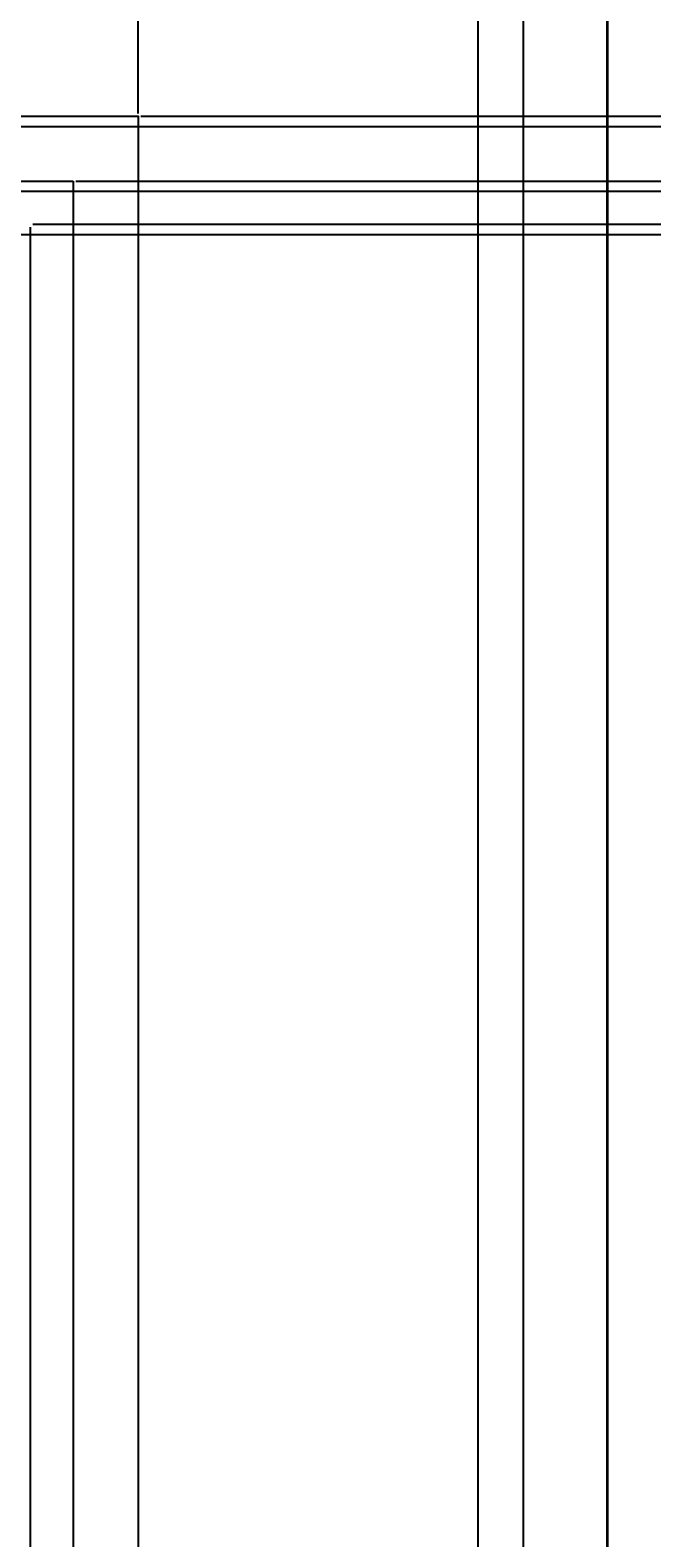
# Model space of a CAD drawing. Units: inches. Extents: x -6 to 289, y -8 to 323.
# Tile 72 of 107: x 234 to 248, y 194 to 229. Entities that reach past the tile are written whole.
import ezdxf

# ---------------------------------------------------------------- set-up
doc = ezdxf.new("R2010")
doc.units = ezdxf.units.IN
doc.header["$MEASUREMENT"] = 0
for name, color, linetype, lineweight in [('A-ANNO-DIMS', 2, 'Continuous', 18), ('A-ELEV', 7, 'Continuous', 35), ('A-GLAZ', 4, 'Continuous', 25)]:
    doc.layers.add(name, color=color, linetype=linetype, lineweight=lineweight)
doc.styles.get("Standard").update_dxf_attribs({"font": 'arial.ttf'})
doc.dimstyles.get("Standard").update_dxf_attribs({"dimtxt": 0.18, "dimasz": 0.18, "dimexe": 0.18, "dimexo": 0.0625, "dimgap": 0.09, "dimtad": 0, "dimtih": 1, "dimtoh": 1, "dimdec": 4, "dimzin": 0, "dimdsep": 46, "dimtxsty": 'Standard', "dimcen": 0.09, "dimadec": 0, "dimazin": 0, "dimtfac": 1, "dimtdec": 4, "dimtofl": 0, "dimtmove": 0, "dimatfit": 3, "dimfxl": 1, "dimtolj": 1, "dimtzin": 0, "dimarcsym": 0})

# ---------------------------------------------------------------- blocks, each defined once
blk = doc.blocks.new('*D13')
at = {"layer": 'A-ANNO-DIMS', "color": 0, "lineweight": -2, "transparency": 16777216}
for p, q in [((188.292, 226.951), (188.292, 322.969)), ((236.292, 226.951), (236.292, 322.969)), ((188.472, 322.789), (212.069, 322.789)), ((236.112, 322.789), (212.515, 322.789))]:
    blk.add_line(p, q, dxfattribs=at)
at = {"layer": 'A-ANNO-DIMS', "color": 0, "transparency": 16777216}
for points in [[(188.472, 322.819), (188.472, 322.759), (188.292, 322.789)], [(236.112, 322.819), (236.112, 322.759), (236.292, 322.789)]]:
    blk.add_solid(points, dxfattribs=at)
at = {"layer": 'Defpoints', "color": 0, "transparency": 16777216}
for p in [(236.292, 322.789), (188.292, 226.889), (236.292, 226.889)]:
    blk.add_point(p, dxfattribs=at)
at = {"layer": 'A-ANNO-DIMS', "color": 0, "transparency": 16777216, "insert": (212.292, 322.789), "char_height": 0.18, "attachment_point": 5}
blk.add_mtext('\\A1;48', dxfattribs=at)
blk = doc.blocks.new('*D14')
at = {"layer": 'A-ANNO-DIMS', "color": 0, "lineweight": -2, "transparency": 16777216}
for p, q in [((236.292, 226.951), (236.292, 322.969)), ((247.164, 162.411), (247.164, 322.969)), ((236.472, 322.789), (241.274, 322.789)), ((246.984, 322.789), (242.182, 322.789))]:
    blk.add_line(p, q, dxfattribs=at)
at = {"layer": 'A-ANNO-DIMS', "color": 0, "transparency": 16777216}
for points in [[(236.472, 322.819), (236.472, 322.759), (236.292, 322.789)], [(246.984, 322.819), (246.984, 322.759), (247.164, 322.789)]]:
    blk.add_solid(points, dxfattribs=at)
at = {"layer": 'Defpoints', "color": 0, "transparency": 16777216}
for p in [(247.164, 322.789), (236.292, 226.889), (247.164, 162.348)]:
    blk.add_point(p, dxfattribs=at)
at = {"layer": 'A-ANNO-DIMS', "color": 0, "transparency": 16777216, "insert": (241.728, 322.789), "char_height": 0.18, "attachment_point": 5}
blk.add_mtext('\\A1;10.872', dxfattribs=at)
blk = doc.blocks.new('*D15')
at = {"layer": 'A-ANNO-DIMS', "color": 0, "lineweight": -2, "transparency": 16777216}
for p, q in [((247.164, 162.411), (247.164, 322.969)), ((271.164, 7.351), (271.164, 322.969)), ((247.344, 322.789), (258.944, 322.789)), ((270.984, 322.789), (259.384, 322.789))]:
    blk.add_line(p, q, dxfattribs=at)
at = {"layer": 'A-ANNO-DIMS', "color": 0, "transparency": 16777216}
for points in [[(247.344, 322.819), (247.344, 322.759), (247.164, 322.789)], [(270.984, 322.819), (270.984, 322.759), (271.164, 322.789)]]:
    blk.add_solid(points, dxfattribs=at)
at = {"layer": 'Defpoints', "color": 0, "transparency": 16777216}
for p in [(271.164, 322.789), (247.164, 162.348), (271.164, 7.289)]:
    blk.add_point(p, dxfattribs=at)
at = {"layer": 'A-ANNO-DIMS', "color": 0, "transparency": 16777216, "insert": (259.164, 322.789), "char_height": 0.18, "attachment_point": 5}
blk.add_mtext('\\A1;24', dxfattribs=at)
blk = doc.blocks.new('*D25')
at = {"layer": 'A-ANNO-DIMS', "color": 0, "lineweight": -2, "transparency": 16777216}
for p, q in [((126.946, 226.654), (288.653, 226.654)), ((288.473, 226.474), (288.473, 202.836)), ((288.473, 178.834), (288.473, 202.472)), ((126.946, 178.654), (288.653, 178.654))]:
    blk.add_line(p, q, dxfattribs=at)
at = {"layer": 'A-ANNO-DIMS', "color": 0, "transparency": 16777216}
for points in [[(288.443, 226.474), (288.503, 226.474), (288.473, 226.654)], [(288.443, 178.834), (288.503, 178.834), (288.473, 178.654)]]:
    blk.add_solid(points, dxfattribs=at)
at = {"layer": 'Defpoints', "color": 0, "transparency": 16777216}
for p in [(126.883, 226.654), (288.473, 226.654), (126.883, 178.654)]:
    blk.add_point(p, dxfattribs=at)
at = {"layer": 'A-ANNO-DIMS', "color": 0, "transparency": 16777216, "insert": (288.473, 202.654), "char_height": 0.18, "attachment_point": 5}
blk.add_mtext('\\A1;48', dxfattribs=at)
blk = doc.blocks.new('*D26')
at = {"layer": 'A-ANNO-DIMS', "color": 0, "lineweight": -2, "transparency": 16777216}
for p, q in [((247.226, 247.289), (288.653, 247.289)), ((288.473, 247.109), (288.473, 237.153)), ((288.473, 226.834), (288.473, 236.789)), ((126.946, 226.654), (288.653, 226.654))]:
    blk.add_line(p, q, dxfattribs=at)
at = {"layer": 'A-ANNO-DIMS', "color": 0, "transparency": 16777216}
for points in [[(288.443, 247.109), (288.503, 247.109), (288.473, 247.289)], [(288.443, 226.834), (288.503, 226.834), (288.473, 226.654)]]:
    blk.add_solid(points, dxfattribs=at)
at = {"layer": 'Defpoints', "color": 0, "transparency": 16777216}
for p in [(247.164, 247.289), (288.473, 247.289), (126.883, 226.654)]:
    blk.add_point(p, dxfattribs=at)
at = {"layer": 'A-ANNO-DIMS', "color": 0, "transparency": 16777216, "insert": (288.473, 236.971), "char_height": 0.18, "attachment_point": 5}
blk.add_mtext('\\A1;20.635', dxfattribs=at)
blk = doc.blocks.new('*D37')
at = {"layer": 'A-ANNO-DIMS', "color": 0, "lineweight": -2, "transparency": 16777216}
for p, q in [((166.446, 224.154), (288.653, 224.154)), ((288.473, 223.974), (288.473, 202.836)), ((288.473, 181.334), (288.473, 202.472)), ((166.446, 181.154), (288.653, 181.154))]:
    blk.add_line(p, q, dxfattribs=at)
at = {"layer": 'A-ANNO-DIMS', "color": 0, "transparency": 16777216}
for points in [[(288.443, 223.974), (288.503, 223.974), (288.473, 224.154)], [(288.443, 181.334), (288.503, 181.334), (288.473, 181.154)]]:
    blk.add_solid(points, dxfattribs=at)
at = {"layer": 'Defpoints', "color": 0, "transparency": 16777216}
for p in [(166.383, 224.154), (288.473, 224.154), (166.383, 181.154)]:
    blk.add_point(p, dxfattribs=at)
at = {"layer": 'A-ANNO-DIMS', "color": 0, "transparency": 16777216, "insert": (288.473, 202.654), "char_height": 0.18, "attachment_point": 5}
blk.add_mtext('\\A1;43', dxfattribs=at)
blk = doc.blocks.new('*D38')
at = {"layer": 'A-ANNO-DIMS', "color": 0, "lineweight": -2, "transparency": 16777216}
for p, q in [((167.446, 225.154), (288.653, 225.154)), ((288.473, 224.974), (288.473, 224.834)), ((288.473, 224.334), (288.473, 224.474)), ((166.446, 224.154), (288.653, 224.154))]:
    blk.add_line(p, q, dxfattribs=at)
at = {"layer": 'A-ANNO-DIMS', "color": 0, "transparency": 16777216}
for points in [[(288.443, 224.974), (288.503, 224.974), (288.473, 225.154)], [(288.443, 224.334), (288.503, 224.334), (288.473, 224.154)]]:
    blk.add_solid(points, dxfattribs=at)
at = {"layer": 'Defpoints', "color": 0, "transparency": 16777216}
for p in [(167.383, 225.154), (288.473, 225.154), (166.383, 224.154)]:
    blk.add_point(p, dxfattribs=at)
at = {"layer": 'A-ANNO-DIMS', "color": 0, "transparency": 16777216, "insert": (288.473, 224.654), "char_height": 0.18, "attachment_point": 5}
blk.add_mtext('\\A1;1', dxfattribs=at)
blk = doc.blocks.new('*D39')
at = {"layer": 'A-ANNO-DIMS', "color": 0, "lineweight": -2, "transparency": 16777216}
for p, q in [((168.946, 226.654), (288.653, 226.654)), ((288.473, 226.474), (288.473, 226.086)), ((288.473, 225.334), (288.473, 225.722)), ((167.446, 225.154), (288.653, 225.154))]:
    blk.add_line(p, q, dxfattribs=at)
at = {"layer": 'A-ANNO-DIMS', "color": 0, "transparency": 16777216}
for points in [[(288.443, 226.474), (288.503, 226.474), (288.473, 226.654)], [(288.443, 225.334), (288.503, 225.334), (288.473, 225.154)]]:
    blk.add_solid(points, dxfattribs=at)
at = {"layer": 'Defpoints', "color": 0, "transparency": 16777216}
for p in [(168.883, 226.654), (288.473, 226.654), (167.383, 225.154)]:
    blk.add_point(p, dxfattribs=at)
at = {"layer": 'A-ANNO-DIMS', "color": 0, "transparency": 16777216, "insert": (288.473, 225.904), "char_height": 0.18, "attachment_point": 5}
blk.add_mtext('\\A1;1.5', dxfattribs=at)
blk = doc.blocks.new('*D44')
at = {"layer": 'A-ANNO-DIMS', "color": 0, "lineweight": -2, "transparency": 16777216}
for p, q in [((212.292, 224.326), (212.292, -8.391)), ((233.792, 224.326), (233.792, -8.391)), ((212.472, -8.211), (222.716, -8.211)), ((233.612, -8.211), (223.368, -8.211))]:
    blk.add_line(p, q, dxfattribs=at)
at = {"layer": 'A-ANNO-DIMS', "color": 0, "transparency": 16777216}
for points in [[(212.472, -8.181), (212.472, -8.241), (212.292, -8.211)], [(233.612, -8.181), (233.612, -8.241), (233.792, -8.211)]]:
    blk.add_solid(points, dxfattribs=at)
at = {"layer": 'Defpoints', "color": 0, "transparency": 16777216}
for p in [(212.292, 224.389), (233.792, 224.389), (233.792, -8.211)]:
    blk.add_point(p, dxfattribs=at)
at = {"layer": 'A-ANNO-DIMS', "color": 0, "transparency": 16777216, "insert": (223.042, -8.211), "char_height": 0.18, "attachment_point": 5}
blk.add_mtext('\\A1;21.5', dxfattribs=at)
blk = doc.blocks.new('*D45')
at = {"layer": 'A-ANNO-DIMS', "color": 0, "lineweight": -2, "transparency": 16777216}
for p, q in [((234.792, 225.326), (234.792, -8.391)), ((233.792, 224.326), (233.792, -8.391)), ((233.972, -8.211), (234.169, -8.211)), ((234.612, -8.211), (234.415, -8.211))]:
    blk.add_line(p, q, dxfattribs=at)
at = {"layer": 'A-ANNO-DIMS', "color": 0, "transparency": 16777216}
for points in [[(233.972, -8.181), (233.972, -8.241), (233.792, -8.211)], [(234.612, -8.181), (234.612, -8.241), (234.792, -8.211)]]:
    blk.add_solid(points, dxfattribs=at)
at = {"layer": 'Defpoints', "color": 0, "transparency": 16777216}
for p in [(234.792, 225.389), (233.792, 224.389), (234.792, -8.211)]:
    blk.add_point(p, dxfattribs=at)
at = {"layer": 'A-ANNO-DIMS', "color": 0, "transparency": 16777216, "insert": (234.292, -8.211), "char_height": 0.18, "attachment_point": 5}
blk.add_mtext('\\A1;1', dxfattribs=at)
blk = doc.blocks.new('*D46')
at = {"layer": 'A-ANNO-DIMS', "color": 0, "lineweight": -2, "transparency": 16777216}
for p, q in [((236.292, 226.826), (236.292, -8.391)), ((234.792, 225.326), (234.792, -8.391)), ((234.972, -8.211), (235.296, -8.211)), ((236.112, -8.211), (235.788, -8.211))]:
    blk.add_line(p, q, dxfattribs=at)
at = {"layer": 'A-ANNO-DIMS', "color": 0, "transparency": 16777216}
for points in [[(234.972, -8.181), (234.972, -8.241), (234.792, -8.211)], [(236.112, -8.181), (236.112, -8.241), (236.292, -8.211)]]:
    blk.add_solid(points, dxfattribs=at)
at = {"layer": 'Defpoints', "color": 0, "transparency": 16777216}
for p in [(236.292, 226.889), (234.792, 225.389), (236.292, -8.211)]:
    blk.add_point(p, dxfattribs=at)
at = {"layer": 'A-ANNO-DIMS', "color": 0, "transparency": 16777216, "insert": (235.542, -8.211), "char_height": 0.18, "attachment_point": 5}
blk.add_mtext('\\A1;1.5', dxfattribs=at)
blk = doc.blocks.new('*D47')
at = {"layer": 'A-ANNO-DIMS', "color": 0, "lineweight": -2, "transparency": 16777216}
for p, q in [((233.854, 224.389), (288.653, 224.389)), ((288.473, 224.209), (288.473, 193.55)), ((288.473, 162.528), (288.473, 193.187)), ((236.354, 162.348), (288.653, 162.348))]:
    blk.add_line(p, q, dxfattribs=at)
at = {"layer": 'A-ANNO-DIMS', "color": 0, "transparency": 16777216}
for points in [[(288.443, 224.209), (288.503, 224.209), (288.473, 224.389)], [(288.443, 162.528), (288.503, 162.528), (288.473, 162.348)]]:
    blk.add_solid(points, dxfattribs=at)
at = {"layer": 'Defpoints', "color": 0, "transparency": 16777216}
for p in [(233.792, 224.389), (288.473, 224.389), (236.292, 162.348)]:
    blk.add_point(p, dxfattribs=at)
at = {"layer": 'A-ANNO-DIMS', "color": 0, "transparency": 16777216, "insert": (288.473, 193.369), "char_height": 0.18, "attachment_point": 5}
blk.add_mtext('\\A1;62.04', dxfattribs=at)
blk = doc.blocks.new('*D48')
at = {"layer": 'A-ANNO-DIMS', "color": 0, "lineweight": -2, "transparency": 16777216}
for p, q in [((234.854, 225.389), (288.653, 225.389)), ((288.473, 225.209), (288.473, 225.069)), ((288.473, 224.569), (288.473, 224.708)), ((233.854, 224.389), (288.653, 224.389))]:
    blk.add_line(p, q, dxfattribs=at)
at = {"layer": 'A-ANNO-DIMS', "color": 0, "transparency": 16777216}
for points in [[(288.443, 225.209), (288.503, 225.209), (288.473, 225.389)], [(288.443, 224.569), (288.503, 224.569), (288.473, 224.389)]]:
    blk.add_solid(points, dxfattribs=at)
at = {"layer": 'Defpoints', "color": 0, "transparency": 16777216}
for p in [(234.792, 225.389), (288.473, 225.389), (233.792, 224.389)]:
    blk.add_point(p, dxfattribs=at)
at = {"layer": 'A-ANNO-DIMS', "color": 0, "transparency": 16777216, "insert": (288.473, 224.889), "char_height": 0.18, "attachment_point": 5}
blk.add_mtext('\\A1;1', dxfattribs=at)
blk = doc.blocks.new('*D49')
at = {"layer": 'A-ANNO-DIMS', "color": 0, "lineweight": -2, "transparency": 16777216}
for p, q in [((236.354, 226.889), (288.653, 226.889)), ((288.473, 226.709), (288.473, 226.321)), ((288.473, 225.569), (288.473, 225.957)), ((234.854, 225.389), (288.653, 225.389))]:
    blk.add_line(p, q, dxfattribs=at)
at = {"layer": 'A-ANNO-DIMS', "color": 0, "transparency": 16777216}
for points in [[(288.443, 226.709), (288.503, 226.709), (288.473, 226.889)], [(288.443, 225.569), (288.503, 225.569), (288.473, 225.389)]]:
    blk.add_solid(points, dxfattribs=at)
at = {"layer": 'Defpoints', "color": 0, "transparency": 16777216}
for p in [(236.292, 226.889), (288.473, 226.889), (234.792, 225.389)]:
    blk.add_point(p, dxfattribs=at)
at = {"layer": 'A-ANNO-DIMS', "color": 0, "transparency": 16777216, "insert": (288.473, 226.139), "char_height": 0.18, "attachment_point": 5}
blk.add_mtext('\\A1;1.5', dxfattribs=at)
blk = doc.blocks.new('*D81')
at = {"layer": 'A-ANNO-DIMS', "color": 0, "lineweight": -2, "transparency": 16777216}
for p, q in [((230.292, 68.842), (230.292, 322.969)), ((245.215, 66.286), (245.215, 322.969)), ((230.472, 322.789), (237.298, 322.789)), ((245.035, 322.789), (238.208, 322.789))]:
    blk.add_line(p, q, dxfattribs=at)
at = {"layer": 'A-ANNO-DIMS', "color": 0, "transparency": 16777216}
for points in [[(230.472, 322.819), (230.472, 322.759), (230.292, 322.789)], [(245.035, 322.819), (245.035, 322.759), (245.215, 322.789)]]:
    blk.add_solid(points, dxfattribs=at)
at = {"layer": 'Defpoints', "color": 0, "transparency": 16777216}
for p in [(245.215, 322.789), (230.292, 68.779), (245.215, 66.224)]:
    blk.add_point(p, dxfattribs=at)
at = {"layer": 'A-ANNO-DIMS', "color": 0, "transparency": 16777216, "insert": (237.753, 322.789), "char_height": 0.18, "attachment_point": 5}
blk.add_mtext('\\A1;14.923', dxfattribs=at)
blk = doc.blocks.new('*D82')
at = {"layer": 'A-ANNO-DIMS', "color": 0, "lineweight": -2, "transparency": 16777216}
for p, q in [((245.215, 66.286), (245.215, 322.969)), ((272.973, 66.286), (272.973, 322.969)), ((245.395, 322.789), (258.699, 322.789)), ((272.793, 322.789), (259.489, 322.789))]:
    blk.add_line(p, q, dxfattribs=at)
at = {"layer": 'A-ANNO-DIMS', "color": 0, "transparency": 16777216}
for points in [[(245.395, 322.819), (245.395, 322.759), (245.215, 322.789)], [(272.793, 322.819), (272.793, 322.759), (272.973, 322.789)]]:
    blk.add_solid(points, dxfattribs=at)
at = {"layer": 'Defpoints', "color": 0, "transparency": 16777216}
for p in [(272.973, 322.789), (245.215, 66.224), (272.973, 66.224)]:
    blk.add_point(p, dxfattribs=at)
at = {"layer": 'A-ANNO-DIMS', "color": 0, "transparency": 16777216, "insert": (259.094, 322.789), "char_height": 0.18, "attachment_point": 5}
blk.add_mtext('\\A1;27.76', dxfattribs=at)
blk = doc.blocks.new('*D98')
at = {"layer": 'A-ANNO-DIMS', "color": 0, "lineweight": -2, "transparency": 16777216}
for p, q in [((202.741, 159.411), (202.741, 322.969)), ((244.164, 159.411), (244.164, 322.969)), ((202.921, 322.789), (223.056, 322.789)), ((243.984, 322.789), (223.849, 322.789))]:
    blk.add_line(p, q, dxfattribs=at)
at = {"layer": 'A-ANNO-DIMS', "color": 0, "transparency": 16777216}
for points in [[(202.921, 322.819), (202.921, 322.759), (202.741, 322.789)], [(243.984, 322.819), (243.984, 322.759), (244.164, 322.789)]]:
    blk.add_solid(points, dxfattribs=at)
at = {"layer": 'Defpoints', "color": 0, "transparency": 16777216}
for p in [(244.164, 322.789), (202.741, 159.348), (244.164, 159.348)]:
    blk.add_point(p, dxfattribs=at)
at = {"layer": 'A-ANNO-DIMS', "color": 0, "transparency": 16777216, "insert": (223.452, 322.789), "char_height": 0.18, "attachment_point": 5}
blk.add_mtext('\\A1;41.42', dxfattribs=at)
blk = doc.blocks.new('*D99')
at = {"layer": 'A-ANNO-DIMS', "color": 0, "lineweight": -2, "transparency": 16777216}
for p, q in [((244.164, 159.411), (244.164, 322.969)), ((247.164, 162.411), (247.164, 322.969)), ((244.344, 322.789), (245.515, 322.789)), ((246.984, 322.789), (245.813, 322.789))]:
    blk.add_line(p, q, dxfattribs=at)
at = {"layer": 'A-ANNO-DIMS', "color": 0, "transparency": 16777216}
for points in [[(244.344, 322.819), (244.344, 322.759), (244.164, 322.789)], [(246.984, 322.819), (246.984, 322.759), (247.164, 322.789)]]:
    blk.add_solid(points, dxfattribs=at)
at = {"layer": 'Defpoints', "color": 0, "transparency": 16777216}
for p in [(247.164, 322.789), (247.164, 162.348), (244.164, 159.348)]:
    blk.add_point(p, dxfattribs=at)
at = {"layer": 'A-ANNO-DIMS', "color": 0, "transparency": 16777216, "insert": (245.664, 322.789), "char_height": 0.18, "attachment_point": 5}
blk.add_mtext('\\A1;3', dxfattribs=at)
blk = doc.blocks.new('*D100')
at = {"layer": 'A-ANNO-DIMS', "color": 0, "lineweight": -2, "transparency": 16777216}
for p, q in [((247.164, 162.411), (247.164, 322.969)), ((259.164, 139.351), (259.164, 322.969)), ((247.344, 322.789), (252.954, 322.789)), ((258.984, 322.789), (253.373, 322.789))]:
    blk.add_line(p, q, dxfattribs=at)
at = {"layer": 'A-ANNO-DIMS', "color": 0, "transparency": 16777216}
for points in [[(247.344, 322.819), (247.344, 322.759), (247.164, 322.789)], [(258.984, 322.819), (258.984, 322.759), (259.164, 322.789)]]:
    blk.add_solid(points, dxfattribs=at)
at = {"layer": 'Defpoints', "color": 0, "transparency": 16777216}
for p in [(259.164, 322.789), (247.164, 162.348), (259.164, 139.289)]:
    blk.add_point(p, dxfattribs=at)
at = {"layer": 'A-ANNO-DIMS', "color": 0, "transparency": 16777216, "insert": (253.164, 322.789), "char_height": 0.18, "attachment_point": 5}
blk.add_mtext('\\A1;12', dxfattribs=at)

msp = doc.modelspace()

# ---------------------------------------------------------------- linework, layer by layer
at = {"layer": 'A-ELEV'}
msp.add_line((247.1638, 139.2888), (247.1638, 247.2888), dxfattribs=at)
at = {"layer": 'A-GLAZ'}
for p, q in [((212.2918, 225.3887), (234.7918, 225.3887)), ((234.7918, 225.3887), (234.7918, 162.3484))]:
    msp.add_line(p, q, dxfattribs=at)
msp.add_lwpolyline([(188.2918, 162.3484), (188.2918, 226.8887), (236.2918, 226.8887), (236.2918, 162.3484)], dxfattribs=at)

# ---------------------------------------------------------------- dimensions: what is measured, and where the dimension line sits
at = {"layer": 'A-ANNO-DIMS'}
for base, p1, p2, override, picture, middle in [((236.2918, 322.7888), (188.2918, 226.8887), (236.2918, 226.8887), {"dimdec": 0, "dimlfac": 1, "dimrnd": 0, "dimzin": 0, "dimdsep": 46, "dimlunit": 2}, '*D13', (212.2918, 322.7888)), ((244.1638, 322.7888), (202.741, 159.3484), (244.1638, 159.3484), {"dimdec": 2, "dimlfac": 1, "dimrnd": 0, "dimzin": 0, "dimdsep": 46, "dimlunit": 2}, '*D98', (223.4524, 322.7888)), ((245.2146, 322.7888), (230.2918, 68.7795), (245.2146, 66.2238), {"dimdec": 3, "dimlfac": 1, "dimrnd": 0, "dimzin": 0, "dimdsep": 46, "dimlunit": 2}, '*D81', (237.7532, 322.7888)), ((247.1638, 322.7888), (236.2918, 226.8887), (247.1638, 162.3484), {"dimdec": 3, "dimlfac": 1, "dimrnd": 0, "dimzin": 0, "dimdsep": 46, "dimlunit": 2}, '*D14', (241.7278, 322.7888)), ((247.1638, 322.7888), (244.1638, 159.3484), (247.1638, 162.3484), {"dimdec": 0, "dimlfac": 1, "dimrnd": 0, "dimzin": 0, "dimdsep": 46, "dimlunit": 2}, '*D99', (245.6638, 322.7888)), ((272.9733, 322.7888), (245.2146, 66.2238), (272.9733, 66.2238), {"dimdec": 2, "dimlfac": 1, "dimrnd": 0, "dimzin": 0, "dimdsep": 46, "dimlunit": 2}, '*D82', (259.0939, 322.7888)), ((271.1638, 322.7888), (247.1638, 162.3484), (271.1638, 7.2888), {"dimdec": 0, "dimlfac": 1, "dimrnd": 0, "dimzin": 0, "dimdsep": 46, "dimlunit": 2}, '*D15', (259.1638, 322.7888)), ((259.1638, 322.7888), (247.1638, 162.3484), (259.1638, 139.2888), {"dimdec": 0, "dimlfac": 1, "dimrnd": 0, "dimzin": 0, "dimdsep": 46, "dimlunit": 2}, '*D100', (253.1638, 322.7888)), ((236.2918, -8.2112), (234.7918, 225.3887), (236.2918, 226.8887), {"dimdec": 1, "dimlfac": 1, "dimrnd": 0, "dimzin": 0, "dimdsep": 46, "dimlunit": 2}, '*D46', (235.5418, -8.2112)), ((234.7918, -8.2112), (233.7918, 224.3887), (234.7918, 225.3887), {"dimdec": 0, "dimlfac": 1, "dimrnd": 0, "dimzin": 0, "dimdsep": 46, "dimlunit": 2}, '*D45', (234.2918, -8.2112)), ((233.7918, -8.2112), (212.2918, 224.3887), (233.7918, 224.3887), {"dimdec": 1, "dimlfac": 1, "dimrnd": 0, "dimzin": 0, "dimdsep": 46, "dimlunit": 2}, '*D44', (223.0418, -8.2112))]:
    dim = msp.add_linear_dim(base=base, p1=p1, p2=p2, dimstyle='Standard', override=override, dxfattribs=at)
    dim.commit()
    dim.dimension.update_dxf_attribs({"geometry": picture, "text_midpoint": middle})
for base, p1, p2, override, picture, middle in [((288.4733, 247.2888), (126.8835, 226.654), (247.1638, 247.2888), {"dimdec": 3, "dimlfac": 1, "dimrnd": 0, "dimzin": 0, "dimdsep": 46, "dimlunit": 2}, '*D26', (288.4733, 236.9714)), ((288.4733, 226.654), (126.8835, 178.654), (126.8835, 226.654), {"dimdec": 0, "dimlfac": 1, "dimrnd": 0, "dimzin": 0, "dimdsep": 46, "dimlunit": 2}, '*D25', (288.4733, 202.654)), ((288.4733, 226.654), (167.3835, 225.154), (168.8835, 226.654), {"dimdec": 1, "dimlfac": 1, "dimrnd": 0, "dimzin": 0, "dimdsep": 46, "dimlunit": 2}, '*D39', (288.4733, 225.904)), ((288.4733, 226.8887), (234.7918, 225.3887), (236.2918, 226.8887), {"dimdec": 1, "dimlfac": 1, "dimrnd": 0, "dimzin": 0, "dimdsep": 46, "dimlunit": 2}, '*D49', (288.4733, 226.1387)), ((288.4733, 225.3887), (233.7918, 224.3887), (234.7918, 225.3887), {"dimdec": 0, "dimlfac": 1, "dimrnd": 0, "dimzin": 0, "dimdsep": 46, "dimlunit": 2}, '*D48', (288.4733, 224.8887)), ((288.4733, 225.154), (166.3835, 224.154), (167.3835, 225.154), {"dimdec": 0, "dimlfac": 1, "dimrnd": 0, "dimzin": 0, "dimdsep": 46, "dimlunit": 2}, '*D38', (288.4733, 224.654)), ((288.4733, 224.3887), (236.2918, 162.3484), (233.7918, 224.3887), {"dimdec": 2, "dimlfac": 1, "dimrnd": 0, "dimzin": 0, "dimdsep": 46, "dimlunit": 2}, '*D47', (288.4733, 193.3685)), ((288.4733, 224.154), (166.3835, 181.154), (166.3835, 224.154), {"dimdec": 0, "dimlfac": 1, "dimrnd": 0, "dimzin": 0, "dimdsep": 46, "dimlunit": 2}, '*D37', (288.4733, 202.654))]:
    dim = msp.add_linear_dim(base=base, p1=p1, p2=p2, angle=90, dimstyle='Standard', override=override, dxfattribs=at)
    dim.commit()
    dim.dimension.update_dxf_attribs({"geometry": picture, "text_midpoint": middle})

doc.saveas('drawing.dxf')
